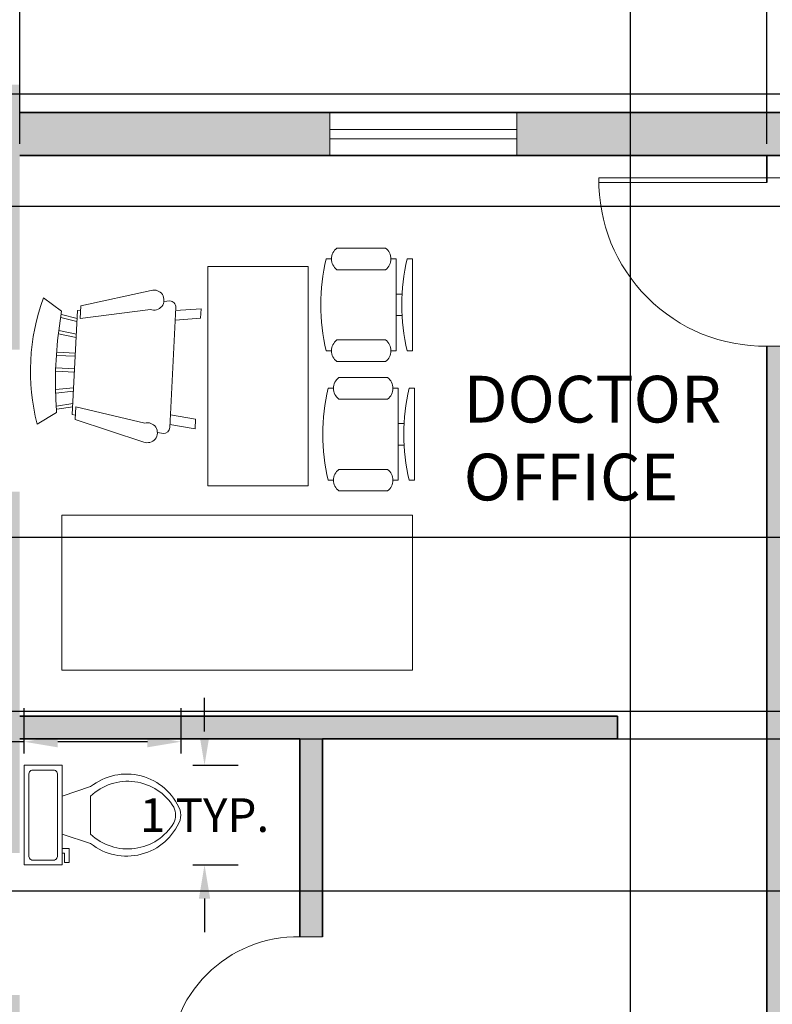
# Model space of a CAD drawing. Units: metres. Extents: x 4298.5 to 4325.2, y 2075 to 2095.8.
# Tile 17 of 35: x 4305.9 to 4309.9, y 2080.5 to 2085.8. Entities that reach past the tile are written whole.
import ezdxf

# ---------------------------------------------------------------- set-up
doc = ezdxf.new("R2010")
doc.units = ezdxf.units.M
for name, color, linetype, lineweight in [('A-ANNO-DIMS', 2, 'Continuous', 18), ('A-AREA-IDEN', 7, 'Continuous', 18), ('A-DOOR', 3, 'Continuous', 18), ('A-EQPM', 9, 'Continuous', 18), ('A-FLOR-FIXT', 15, 'Continuous', 18), ('A-FURN', 15, 'Continuous', 18), ('A-GLAZ', 4, 'Continuous', 18), ('A-WALL', 7, 'Continuous', 35), ('A-WALL-PATT', 252, 'Continuous', 13)]:
    doc.layers.add(name, color=color, linetype=linetype, lineweight=lineweight)
doc.styles.get("Standard").update_dxf_attribs({"font": 'arial.ttf'})
doc.dimstyles.get("Standard").update_dxf_attribs({"dimtxt": 0.18, "dimasz": 0.18, "dimexe": 0.18, "dimexo": 0.0625, "dimgap": 0.09, "dimtad": 0, "dimtih": 1, "dimtoh": 1, "dimdec": 4, "dimzin": 0, "dimdsep": 46, "dimtxsty": 'Standard', "dimcen": 0.09, "dimadec": 0, "dimazin": 0, "dimtfac": 1, "dimtdec": 4, "dimtofl": 0, "dimtmove": 0, "dimatfit": 3, "dimfxl": 1, "dimtolj": 1, "dimtzin": 0, "dimarcsym": 0})

# ---------------------------------------------------------------- blocks, each defined once
blk = doc.blocks.new('Chair - Desk')
for p, q in [((-8.5, 0), (-8.5, -1)), ((-8.5, 0), (8.5, 0)), ((8.5, 0), (8.5, -1)), ((-8.5, -3), (-8.5, -4)), ((-8.5, -3), (8.5, -3)), ((-2, -3), (-2, -1.9355)), ((2, -1.9576), (2, -3)), ((8.5, -3), (8.5, -4)), ((-10.5, -5), (-10.5, -14)), ((-6.5, -14), (-6.5, -5)), ((6.5, -5), (6.5, -14)), ((10.5, -14), (10.5, -5)), ((-8.5, -15), (-8.5, -16)), ((8.5, -15), (8.5, -16))]:
    blk.add_line(p, q)
for centre, radius, start, end in [((0, 34.625), 36.625, 256.5803, 283.4197), ((-8.5, -6.5), 2.5, 36.8699, 143.1301), ((8.5, -6.5), 2.5, 36.8699, 143.1301), ((-8.5, -12.5), 2.5, 216.8699, 323.1301), ((8.5, -12.5), 2.5, 216.8699, 323.1301), ((0, 19.625), 36.625, 256.5803, 283.4197)]:
    blk.add_arc(centre, radius, start, end)
blk = doc.blocks.new('Chair - Rocking')
for p, q in [((-8, -4.5), (-10, -1.5)), ((8, -4.5), (10, -1.5)), ((-7.5, -4.5), (-7, -7)), ((-6.5, -7), (-7.02225, -4.43)), ((-4.5, -7), (-4.96674, -4.19951)), ((-4, -7), (-4.40532, -4.16272)), ((-1.5, -4.05012), (-1.5, -7)), ((-1, -7), (-1, -4.05012)), ((1, -7), (1, -4.04655)), ((1.5, -4.05012), (1.5, -7)), ((4, -7), (4.40187, -4.18694)), ((4.5, -7), (4.96761, -4.19437)), ((6.5, -7), (7, -4.4057)), ((7.5, -4.5), (7, -7)), ((-9, -7.5), (-12, -18.49999)), ((-7, -7.5), (-9, -7.5)), ((-9, -18.49999), (-7, -7.5)), ((-8.23428, -6.99939), (-8.3093, -7.47958)), ((-8.23041, -7), (8.23915, -7)), ((7, -7.5), (9, -7.5)), ((9, -18.49999), (7, -7.5)), ((8.31071, -7.48854), (8.23449, -7.00073)), ((9, -7.5), (12, -18.49999)), ((-10.36644, -20.64523), (-10.5, -21.49999)), ((10.5, -21.49999), (10.3575, -20.58798)), ((-9, -22.49999), (-9.5, -26.49999)), ((0, -22.49999), (-9.5, -22.49999)), ((-8, -26.49999), (-7.5, -22.49999)), ((0, -22.49999), (9.5, -22.49999)), ((8, -26.49999), (7.5, -22.49999)), ((9, -22.49999), (9.5, -26.49999)), ((-9.5, -26.49999), (-8, -26.49999)), ((9.5, -26.49999), (8, -26.49999))]:
    blk.add_line(p, q)
for centre, radius, start, end in [((0, -34.08333), 34.08333, 72.93847, 107.0615), ((0, -68.25004), 64.25, 93.92211, 97.15267), ((0, -68.25004), 64.25, 82.84733, 93.92211), ((-10.5, -18.99999), 1.58114, 161.5651, 18.43495), ((10.5, -18.99999), 1.58114, 161.5651, 18.43495), ((-9.5, -21.49999), 1, 180, 270), ((9.5, -21.49999), 1, 270, 0)]:
    blk.add_arc(centre, radius, start, end)
blk = doc.blocks.new('Toilet - top')
for p, q in [((9.5, -6), (9.5, -2)), ((-8, -8.5), (-8, -8)), ((-7, -8), (-7, -9.5)), ((-4, -8), (-6, -14)), ((4, -8), (6, -14)), ((-10, -8.5), (-8, -8.5)), ((-10, -9.5), (-10, -8.5)), ((-7, -9.5), (-10, -9.5)), ((4, -14), (-4, -14))]:
    blk.add_line(p, q)
blk.add_lwpolyline([(10.5, -8), (10.5, 0), (-10.5, 0), (-10.5, -8)], close=True)
for points in [[(-9.5, -2), (-9.5, -6)], [(8.5, -1), (-8.5, -1)], [(-8.5, -7), (8.5, -7)]]:
    blk.add_lwpolyline(points)
for centre, radius, start, end in [((-8.62, -1.88), 0.884, 81.8699, 188.1301), ((8.62, -1.88), 0.884, 351.8699, 98.1301), ((-8.62, -6.12), 0.884, 171.8699, 278.1301), ((8.62, -6.12), 0.884, 261.8699, 8.1301), ((3.52, -21.58), 12.17, 141.4691, 247.9714), ((4.2, -21.82), 11.33, 136.3677, 238.9468), ((-3.52, -21.58), 12.17, 292.0284, 38.5307), ((-4.2, -21.82), 11.33, 301.053, 43.6321), ((0, -27.88), 4, 245.7318, 294.2682), ((0, -29), 4, 254.8605, 285.1395)]:
    blk.add_arc(centre, radius, start, end)
blk = doc.blocks.new('WIN-1000-GLASS')
for p, q in [((1, 0.05), (0, 0.05)), ((1, 0), (0, 0))]:
    blk.add_line(p, q)
blk = doc.blocks.new('DOOR-900-LEAF')
for p, q in [((0.9, 0.9), (0, 0.9)), ((0.9, 0.875), (0, 0.875))]:
    blk.add_line(p, q)
blk.add_arc((0.8875, 0.8875), 0.8876, 179.1931, 270.8069)
blk = doc.blocks.new('DOOR-700-LEAF')
for p, q in [((0.675, 0), (0.675, 0.7)), ((0.7, 0), (0.7, 0.7))]:
    blk.add_line(p, q)
blk.add_arc((0.6875, 0.0125), 0.6876, 88.9584, 181.0416)
blk = doc.blocks.new('DESK-1175')
blk.add_lwpolyline([(0, 1.1735), (0.5376, 1.1735), (0.5376, 0), (0, 0)], close=True)
blk = doc.blocks.new('EXAM-TABLE-1880')
blk.add_lwpolyline([(0, 0.8289), (1.8779, 0.8289), (1.8779, 0), (0, 0)], close=True)
blk = doc.blocks.new('*D31')
at = {"layer": 'A-ANNO-DIMS', "color": 0, "lineweight": -2, "transparency": 16777216}
for p, q in [((4305.9147, 2081.8585), (4305.9147, 2082.1019)), ((4306.7541, 2081.8585), (4306.7541, 2082.1019)), ((4305.9147, 2081.9219), (4305.7347, 2081.9219)), ((4306.5741, 2081.9219), (4306.0947, 2081.9219))]:
    blk.add_line(p, q, dxfattribs=at)
at = {"layer": 'A-ANNO-DIMS', "color": 0, "transparency": 16777216}
for points in [[(4306.0947, 2081.9519), (4306.0947, 2081.8919), (4305.9147, 2081.9219)], [(4306.5741, 2081.9519), (4306.5741, 2081.8919), (4306.7541, 2081.9219)]]:
    blk.add_solid(points, dxfattribs=at)
at = {"layer": 'Defpoints', "color": 0, "transparency": 16777216}
for p in [(4305.9147, 2081.9219), (4305.9147, 2081.796), (4306.7541, 2081.796)]:
    blk.add_point(p, dxfattribs=at)
at = {"layer": 'A-ANNO-DIMS', "color": 0, "transparency": 16777216, "insert": (4305.0285, 2081.9219), "char_height": 0.18, "attachment_point": 5}
blk.add_mtext('\\A1;WC 1 TYP.', dxfattribs=at)
blk = doc.blocks.new('*D32')
at = {"layer": 'A-ANNO-DIMS', "color": 0, "lineweight": -2, "transparency": 16777216}
for p, q in [((4306.88, 2081.976), (4306.88, 2082.156)), ((4306.8166, 2081.796), (4307.06, 2081.796)), ((4306.8166, 2081.2626), (4307.06, 2081.2626)), ((4306.88, 2081.0826), (4306.88, 2080.9026))]:
    blk.add_line(p, q, dxfattribs=at)
at = {"layer": 'A-ANNO-DIMS', "color": 0, "transparency": 16777216}
for points in [[(4306.85, 2081.976), (4306.91, 2081.976), (4306.88, 2081.796)], [(4306.85, 2081.0826), (4306.91, 2081.0826), (4306.88, 2081.2626)]]:
    blk.add_solid(points, dxfattribs=at)
at = {"layer": 'Defpoints', "color": 0, "transparency": 16777216}
for p in [(4306.7541, 2081.796), (4306.88, 2081.796), (4306.7541, 2081.2626)]:
    blk.add_point(p, dxfattribs=at)
at = {"layer": 'A-ANNO-DIMS', "color": 0, "transparency": 16777216, "insert": (4306.88, 2081.5293), "char_height": 0.18, "attachment_point": 5}
blk.add_mtext('\\A1;1 TYP.', dxfattribs=at)
blk = doc.blocks.new('*D47')
at = {"layer": 'A-ANNO-DIMS', "color": 0, "lineweight": -2, "transparency": 16777216}
for p, q in [((4300.4306, 2084.4956), (4300.4306, 2074.9896)), ((4322.8106, 2084.4956), (4322.8106, 2074.9896)), ((4300.6106, 2075.1696), (4311.2252, 2075.1696)), ((4322.6306, 2075.1696), (4312.016, 2075.1696))]:
    blk.add_line(p, q, dxfattribs=at)
at = {"layer": 'A-ANNO-DIMS', "color": 0, "transparency": 16777216}
for points in [[(4300.6106, 2075.1996), (4300.6106, 2075.1396), (4300.4306, 2075.1696)], [(4322.6306, 2075.1996), (4322.6306, 2075.1396), (4322.8106, 2075.1696)]]:
    blk.add_solid(points, dxfattribs=at)
at = {"layer": 'Defpoints', "color": 0, "transparency": 16777216}
for p in [(4300.4306, 2084.5581), (4322.8106, 2084.5581), (4322.8106, 2075.1696)]:
    blk.add_point(p, dxfattribs=at)
at = {"layer": 'A-ANNO-DIMS', "color": 0, "transparency": 16777216, "insert": (4311.6206, 2075.1696), "char_height": 0.18, "attachment_point": 5}
blk.add_mtext('\\A1;22.38', dxfattribs=at)
blk = doc.blocks.new('*D53')
at = {"layer": 'A-ANNO-DIMS', "color": 0, "lineweight": -2, "transparency": 16777216}
for p, q in [((4309.1606, 2076.3906), (4309.1606, 2095.8166)), ((4316.8106, 2076.3906), (4316.8106, 2095.8166)), ((4309.3406, 2095.6366), (4312.6619, 2095.6366)), ((4316.6306, 2095.6366), (4313.3093, 2095.6366))]:
    blk.add_line(p, q, dxfattribs=at)
at = {"layer": 'A-ANNO-DIMS', "color": 0, "transparency": 16777216}
for points in [[(4309.3406, 2095.6666), (4309.3406, 2095.6066), (4309.1606, 2095.6366)], [(4316.6306, 2095.6666), (4316.6306, 2095.6066), (4316.8106, 2095.6366)]]:
    blk.add_solid(points, dxfattribs=at)
at = {"layer": 'Defpoints', "color": 0, "transparency": 16777216}
for p in [(4316.8106, 2095.6366), (4309.1606, 2076.3281), (4316.8106, 2076.3281)]:
    blk.add_point(p, dxfattribs=at)
at = {"layer": 'A-ANNO-DIMS', "color": 0, "transparency": 16777216, "insert": (4312.9856, 2095.6366), "char_height": 0.18, "attachment_point": 5}
blk.add_mtext('\\A1;7.65', dxfattribs=at)
blk = doc.blocks.new('*D56')
at = {"layer": 'A-ANNO-DIMS', "color": 0, "lineweight": -2, "transparency": 16777216}
for p, q in [((4305.8281, 2085.0581), (4299.0921, 2085.0581)), ((4299.2721, 2084.8781), (4299.2721, 2083.74)), ((4299.2721, 2082.2381), (4299.2721, 2083.3761)), ((4305.8281, 2082.0581), (4299.0921, 2082.0581))]:
    blk.add_line(p, q, dxfattribs=at)
at = {"layer": 'A-ANNO-DIMS', "color": 0, "transparency": 16777216}
for points in [[(4299.2421, 2084.8781), (4299.3021, 2084.8781), (4299.2721, 2085.0581)], [(4299.2421, 2082.2381), (4299.3021, 2082.2381), (4299.2721, 2082.0581)]]:
    blk.add_solid(points, dxfattribs=at)
at = {"layer": 'Defpoints', "color": 0, "transparency": 16777216}
for p in [(4299.2721, 2085.0581), (4305.8906, 2085.0581), (4305.8906, 2082.0581)]:
    blk.add_point(p, dxfattribs=at)
at = {"layer": 'A-ANNO-DIMS', "color": 0, "transparency": 16777216, "insert": (4299.2721, 2083.5581), "char_height": 0.18, "attachment_point": 5}
blk.add_mtext('\\A1;3', dxfattribs=at)
blk = doc.blocks.new('*D57')
at = {"layer": 'A-ANNO-DIMS', "color": 0, "lineweight": -2, "transparency": 16777216}
for p, q in [((4305.8906, 2085.1206), (4305.8906, 2095.8166)), ((4309.8906, 2085.1206), (4309.8906, 2095.8166)), ((4306.0706, 2095.6366), (4307.7383, 2095.6366)), ((4309.7106, 2095.6366), (4308.0428, 2095.6366))]:
    blk.add_line(p, q, dxfattribs=at)
at = {"layer": 'A-ANNO-DIMS', "color": 0, "transparency": 16777216}
for points in [[(4306.0706, 2095.6666), (4306.0706, 2095.6066), (4305.8906, 2095.6366)], [(4309.7106, 2095.6666), (4309.7106, 2095.6066), (4309.8906, 2095.6366)]]:
    blk.add_solid(points, dxfattribs=at)
at = {"layer": 'Defpoints', "color": 0, "transparency": 16777216}
for p in [(4309.8906, 2095.6366), (4305.8906, 2085.0581), (4309.8906, 2085.0581)]:
    blk.add_point(p, dxfattribs=at)
at = {"layer": 'A-ANNO-DIMS', "color": 0, "transparency": 16777216, "insert": (4307.8906, 2095.6366), "char_height": 0.18, "attachment_point": 5}
blk.add_mtext('\\A1;4', dxfattribs=at)
blk = doc.blocks.new('*D58')
at = {"layer": 'A-ANNO-DIMS', "color": 0, "lineweight": -2, "transparency": 16777216}
for p, q in [((4324.5871, 2085.3881), (4324.5871, 2085.5681)), ((4324.5871, 2085.5681), (4324.7671, 2085.5681)), ((4300.7231, 2085.3881), (4324.7671, 2085.3881)), ((4324.5871, 2084.9681), (4324.5871, 2085.2081)), ((4300.7231, 2084.7881), (4324.7671, 2084.7881))]:
    blk.add_line(p, q, dxfattribs=at)
at = {"layer": 'A-ANNO-DIMS', "color": 0, "transparency": 16777216}
for points in [[(4324.5571, 2085.2081), (4324.6171, 2085.2081), (4324.5871, 2085.3881)], [(4324.5571, 2084.9681), (4324.6171, 2084.9681), (4324.5871, 2084.7881)]]:
    blk.add_solid(points, dxfattribs=at)
at = {"layer": 'Defpoints', "color": 0, "transparency": 16777216}
for p in [(4300.6606, 2085.3881), (4324.5871, 2085.3881), (4300.6606, 2084.7881)]:
    blk.add_point(p, dxfattribs=at)
at = {"layer": 'A-ANNO-DIMS', "color": 0, "transparency": 16777216, "insert": (4325.0209, 2085.5681), "char_height": 0.18, "attachment_point": 5}
blk.add_mtext('\\A1;0.6', dxfattribs=at)
blk = doc.blocks.new('*D60')
at = {"layer": 'A-ANNO-DIMS', "color": 0, "lineweight": -2, "transparency": 16777216}
for p, q in [((4305.9531, 2081.9381), (4324.7671, 2081.9381)), ((4324.5871, 2081.7581), (4324.5871, 2081.18)), ((4324.5871, 2080.2381), (4324.5871, 2080.8162)), ((4305.9531, 2080.0581), (4324.7671, 2080.0581))]:
    blk.add_line(p, q, dxfattribs=at)
at = {"layer": 'A-ANNO-DIMS', "color": 0, "transparency": 16777216}
for points in [[(4324.5571, 2081.7581), (4324.6171, 2081.7581), (4324.5871, 2081.9381)], [(4324.5571, 2080.2381), (4324.6171, 2080.2381), (4324.5871, 2080.0581)]]:
    blk.add_solid(points, dxfattribs=at)
at = {"layer": 'Defpoints', "color": 0, "transparency": 16777216}
for p in [(4305.8906, 2081.9381), (4324.5871, 2081.9381), (4305.8906, 2080.0581)]:
    blk.add_point(p, dxfattribs=at)
at = {"layer": 'A-ANNO-DIMS', "color": 0, "transparency": 16777216, "insert": (4324.5871, 2080.9981), "char_height": 0.18, "attachment_point": 5}
blk.add_mtext('\\A1;1.88', dxfattribs=at)
blk = doc.blocks.new('*D62')
at = {"layer": 'A-ANNO-DIMS', "color": 0, "lineweight": -2, "transparency": 16777216}
for p, q in [((4312.1097, 2083.0153), (4299.0921, 2083.0153)), ((4299.2721, 2082.8353), (4299.2721, 2082.7313)), ((4299.2721, 2082.2635), (4299.2721, 2082.3674)), ((4312.1097, 2082.0835), (4299.0921, 2082.0835))]:
    blk.add_line(p, q, dxfattribs=at)
at = {"layer": 'A-ANNO-DIMS', "color": 0, "transparency": 16777216}
for points in [[(4299.2421, 2082.8353), (4299.3021, 2082.8353), (4299.2721, 2083.0153)], [(4299.2421, 2082.2635), (4299.3021, 2082.2635), (4299.2721, 2082.0835)]]:
    blk.add_solid(points, dxfattribs=at)
at = {"layer": 'Defpoints', "color": 0, "transparency": 16777216}
for p in [(4312.1722, 2083.0153), (4299.2721, 2082.0835), (4312.1722, 2082.0835)]:
    blk.add_point(p, dxfattribs=at)
at = {"layer": 'A-ANNO-DIMS', "color": 0, "transparency": 16777216, "insert": (4299.2721, 2082.5494), "char_height": 0.18, "attachment_point": 5}
blk.add_mtext('\\A1;0.93', dxfattribs=at)
blk = doc.blocks.new('*D63')
at = {"layer": 'A-ANNO-DIMS', "color": 0, "lineweight": -2, "transparency": 16777216}
for p, q in [((4312.1097, 2082.0835), (4299.0921, 2082.0835)), ((4299.2721, 2081.9035), (4299.2721, 2081.7847)), ((4299.2721, 2081.3021), (4299.2721, 2081.4209)), ((4312.1097, 2081.1221), (4299.0921, 2081.1221))]:
    blk.add_line(p, q, dxfattribs=at)
at = {"layer": 'A-ANNO-DIMS', "color": 0, "transparency": 16777216}
for points in [[(4299.2421, 2081.9035), (4299.3021, 2081.9035), (4299.2721, 2082.0835)], [(4299.2421, 2081.3021), (4299.3021, 2081.3021), (4299.2721, 2081.1221)]]:
    blk.add_solid(points, dxfattribs=at)
at = {"layer": 'Defpoints', "color": 0, "transparency": 16777216}
for p in [(4312.1722, 2082.0835), (4299.2721, 2081.1221), (4312.1722, 2081.1221)]:
    blk.add_point(p, dxfattribs=at)
at = {"layer": 'A-ANNO-DIMS', "color": 0, "transparency": 16777216, "insert": (4299.2721, 2081.6028), "char_height": 0.18, "attachment_point": 5}
blk.add_mtext('\\A1;0.96', dxfattribs=at)
blk = doc.blocks.new('*D64')
at = {"layer": 'A-ANNO-DIMS', "color": 0, "lineweight": -2, "transparency": 16777216}
for p, q in [((4312.1097, 2081.1221), (4299.0921, 2081.1221)), ((4299.2721, 2080.9421), (4299.2721, 2080.427)), ((4312.1097, 2080.247), (4299.0921, 2080.247)), ((4299.2721, 2080.247), (4299.2721, 2080.067)), ((4299.2721, 2080.067), (4299.0921, 2080.067))]:
    blk.add_line(p, q, dxfattribs=at)
at = {"layer": 'A-ANNO-DIMS', "color": 0, "transparency": 16777216}
for points in [[(4299.2421, 2080.9421), (4299.3021, 2080.9421), (4299.2721, 2081.1221)], [(4299.2421, 2080.427), (4299.3021, 2080.427), (4299.2721, 2080.247)]]:
    blk.add_solid(points, dxfattribs=at)
at = {"layer": 'Defpoints', "color": 0, "transparency": 16777216}
for p in [(4312.1722, 2081.1221), (4299.2721, 2080.247), (4312.1722, 2080.247)]:
    blk.add_point(p, dxfattribs=at)
at = {"layer": 'A-ANNO-DIMS', "color": 0, "transparency": 16777216, "insert": (4298.7681, 2080.067), "char_height": 0.18, "attachment_point": 5}
blk.add_mtext('\\A1;0.88', dxfattribs=at)

msp = doc.modelspace()

# ---------------------------------------------------------------- hatches: boundary and pattern name
at = {"layer": 'A-WALL-PATT'}
h = msp.add_hatch(color=256, dxfattribs=at)
h.dxf.hatch_style = 1
h.paths.add_polyline_path([(4308.7606, 2094.4781), (4308.1606, 2094.4781), (4307.4606, 2094.4781), (4307.4606, 2094.2481), (4308.2706, 2094.2481), (4308.2706, 2094.1281), (4308.3906, 2094.1281), (4308.3906, 2094.2481), (4308.7606, 2094.2481)])
h.paths.add_polyline_path([(4310.1206, 2094.4781), (4309.5206, 2094.4781), (4309.5206, 2094.2481), (4309.8906, 2094.2481), (4309.8906, 2092.2481), (4308.3906, 2092.2481), (4308.3906, 2093.4281), (4308.2706, 2093.4281), (4308.2706, 2092.0181), (4309.8906, 2092.0181), (4309.8906, 2087.0181), (4309.7706, 2087.0181), (4309.7706, 2086.7881), (4309.8906, 2086.7881), (4311.9406, 2086.7881), (4311.9406, 2087.0181), (4310.1206, 2087.0181), (4310.1206, 2089.0181), (4310.2406, 2089.0181), (4310.2406, 2089.1381), (4310.1206, 2089.1381), (4310.1206, 2092.0181), (4310.3078, 2092.0181), (4310.3078, 2092.2481), (4310.1206, 2092.2481)])
h.paths.add_polyline_path([(4311.7406, 2092.2481), (4311.0678, 2092.2481), (4311.0678, 2092.0181), (4311.7406, 2092.0181)], flags=17)
h.paths.add_polyline_path([(4313.1733, 2092.2481), (4312.5006, 2092.2481), (4312.5006, 2092.0181), (4313.1733, 2092.0181)])
h.paths.add_polyline_path([(4314.5378, 2092.2481), (4314.1206, 2092.2481), (4313.9333, 2092.2481), (4313.9333, 2092.0181), (4314.1206, 2092.0181), (4314.1206, 2087.0181), (4314.0006, 2087.0181), (4314.0006, 2086.7881), (4314.1206, 2086.7881), (4315.5718, 2086.7881), (4315.5718, 2087.0181), (4314.3506, 2087.0181), (4314.3506, 2092.0181), (4314.5378, 2092.0181)])
h.paths.add_polyline_path([(4315.9706, 2092.2481), (4315.2978, 2092.2481), (4315.2978, 2092.0181), (4315.9706, 2092.0181)])
h.paths.add_polyline_path([(4317.4033, 2092.2481), (4316.7306, 2092.2481), (4316.7306, 2092.0181), (4317.4033, 2092.0181)])
h.paths.add_polyline_path([(4318.9506, 2092.2481), (4318.3506, 2092.2481), (4318.1633, 2092.2481), (4318.1633, 2092.0181), (4318.3506, 2092.0181), (4318.3506, 2091.8981), (4318.5806, 2091.8981), (4318.5806, 2092.0181), (4318.9506, 2092.0181)])
h.paths.add_polyline_path([(4321.0106, 2092.2481), (4319.7106, 2092.2481), (4319.7106, 2092.0181), (4320.0806, 2092.0181), (4320.0806, 2090.0181), (4318.5806, 2090.0181), (4318.5806, 2091.1981), (4318.3506, 2091.1981), (4318.3506, 2090.0181), (4318.3506, 2087.0181), (4318.2306, 2087.0181), (4318.2306, 2086.7881), (4318.3506, 2086.7881), (4318.3506, 2086.3081), (4318.5806, 2086.3081), (4318.5806, 2089.7881), (4321.7806, 2089.7881), (4321.7806, 2090.0181), (4320.2006, 2090.0181), (4320.2006, 2092.0181), (4321.0106, 2092.0181)])
h.paths.add_polyline_path([(4322.8106, 2092.2481), (4321.7706, 2092.2481), (4321.7706, 2092.0181), (4322.5806, 2092.0181), (4322.5806, 2091.2831), (4322.8106, 2091.2831)])
h.paths.add_polyline_path([(4322.8106, 2090.5231), (4322.5806, 2090.5231), (4322.5806, 2089.7881), (4322.5806, 2089.5254), (4322.8106, 2089.5254), (4322.8106, 2090.0181)])
h.paths.add_polyline_path([(4322.8106, 2088.7654), (4322.5806, 2088.7654), (4322.5806, 2087.6681), (4322.8106, 2087.6681)])
h.paths.add_polyline_path([(4322.8106, 2086.9081), (4322.5806, 2086.9081), (4322.5806, 2085.8107), (4322.8106, 2085.8107)])
h.paths.add_polyline_path([(4322.8106, 2085.0507), (4322.5806, 2085.0507), (4322.5806, 2084.7881), (4318.5806, 2084.7881), (4318.5806, 2085.0581), (4318.5806, 2085.4081), (4318.3506, 2085.4081), (4318.3506, 2084.5581), (4318.3506, 2080.8581), (4318.4706, 2080.8581), (4318.4706, 2082.3281), (4319.2606, 2082.3281), (4319.2606, 2082.5581), (4318.5806, 2082.5581), (4318.5806, 2084.5581), (4320.0806, 2084.5581), (4320.0806, 2083.9381), (4320.3106, 2083.9381), (4320.3106, 2084.5581), (4322.8106, 2084.5581)])
h.paths.add_polyline_path([(4320.3106, 2083.1781), (4320.0806, 2083.1781), (4320.0806, 2082.5581), (4319.9606, 2082.5581), (4319.9606, 2082.3281), (4320.0806, 2082.3281), (4320.0806, 2081.5731), (4320.3106, 2081.5731)], flags=17)
h.paths.add_polyline_path([(4320.3106, 2080.8131), (4320.0806, 2080.8131), (4320.0806, 2080.0581), (4318.4286, 2080.0581), (4318.4286, 2079.8281), (4320.3106, 2079.8281)])
h.paths.add_polyline_path([(4317.3506, 2085.2881), (4316.5718, 2085.2881), (4316.5718, 2085.0581), (4317.3506, 2085.0581)])
h.paths.add_polyline_path([(4315.5718, 2085.2881), (4314.8434, 2085.2881), (4314.8434, 2085.0581), (4315.5718, 2085.0581)])
h.paths.add_polyline_path([(4313.8434, 2085.2881), (4312.9406, 2085.2881), (4312.9406, 2085.0581), (4313.8434, 2085.0581)])
h.paths.add_polyline_path([(4311.9406, 2085.2881), (4311.4406, 2085.2881), (4311.4406, 2085.0581), (4311.9406, 2085.0581)])
h.paths.add_polyline_path([(4317.3306, 2087.0181), (4316.5718, 2087.0181), (4316.5718, 2086.7881), (4317.3306, 2086.7881)])
h.paths.add_polyline_path([(4313.1006, 2089.1381), (4311.1406, 2089.1381), (4311.1406, 2089.0181), (4312.9806, 2089.0181), (4312.9806, 2087.0181), (4312.9406, 2087.0181), (4312.9406, 2086.7881), (4313.1006, 2086.7881), (4313.1006, 2087.0181)])
h.paths.add_polyline_path([(4307.5515, 2087.0181), (4305.8906, 2087.0181), (4305.8906, 2092.2481), (4305.8906, 2094.2481), (4306.7006, 2094.2481), (4306.7006, 2094.4781), (4305.6606, 2094.4781), (4305.6606, 2092.2481), (4305.2906, 2092.2481), (4305.2906, 2092.0181), (4305.6606, 2092.0181), (4305.6606, 2090.0181), (4304.1606, 2090.0181), (4304.1606, 2091.1981), (4304.0406, 2091.1981), (4304.0406, 2089.9081), (4301.5606, 2089.9081), (4301.5606, 2089.7881), (4304.0406, 2089.7881), (4305.6606, 2089.7881), (4305.6606, 2086.6381), (4305.8906, 2086.6381), (4305.8906, 2086.7881), (4307.5515, 2086.7881)])
h.paths.add_polyline_path([(4307.5515, 2085.2881), (4305.8906, 2085.2881), (4305.8906, 2085.4381), (4305.6606, 2085.4381), (4305.6606, 2084.7881), (4305.2906, 2084.7881), (4305.2906, 2084.5581), (4305.6606, 2084.5581), (4305.6606, 2084.02), (4305.8906, 2084.02), (4305.8906, 2084.5581), (4305.8906, 2085.0581), (4307.5515, 2085.0581)])
h.paths.add_polyline_path([(4310.2406, 2085.2881), (4308.5515, 2085.2881), (4308.5515, 2085.0581), (4310.2406, 2085.0581)])
h.paths.add_polyline_path([(4317.4286, 2080.0581), (4316.5718, 2080.0581), (4316.5718, 2079.8281), (4317.4286, 2079.8281)])
h.paths.add_polyline_path([(4315.5718, 2080.0581), (4314.8434, 2080.0581), (4314.8434, 2079.8281), (4315.5718, 2079.8281)])
h.paths.add_polyline_path([(4313.8434, 2080.0581), (4312.9406, 2080.0581), (4312.9406, 2079.8281), (4313.8434, 2079.8281)])
h.paths.add_polyline_path([(4311.9406, 2080.0581), (4311.4406, 2080.0581), (4311.4406, 2079.8281), (4311.9406, 2079.8281)])
h.paths.add_polyline_path([(4310.2406, 2080.0581), (4310.1206, 2080.0581), (4310.1206, 2084.0381), (4309.8906, 2084.0381), (4309.8906, 2080.0581), (4309.1606, 2080.0581), (4309.1606, 2079.8281), (4310.2406, 2079.8281)])
h.paths.add_polyline_path([(4308.1606, 2080.0581), (4307.5106, 2080.0581), (4307.5106, 2080.1781), (4307.3906, 2080.1781), (4307.3906, 2080.0581), (4305.8906, 2080.0581), (4305.8906, 2080.567), (4305.6606, 2080.567), (4305.6606, 2079.8281), (4308.1606, 2079.8281)])
h.paths.add_polyline_path([(4307.5106, 2081.9381), (4309.0906, 2081.9381), (4309.0906, 2082.0581), (4305.8906, 2082.0581), (4305.8906, 2083.26), (4305.6606, 2083.26), (4305.6606, 2081.327), (4305.8906, 2081.327), (4305.8906, 2081.9381), (4307.3906, 2081.9381), (4307.3906, 2080.8781), (4307.5106, 2080.8781)])
h.paths.add_polyline_path([(4304.5306, 2084.7881), (4302.7306, 2084.7881), (4302.7306, 2084.5581), (4304.5306, 2084.5581)])
h.paths.add_polyline_path([(4301.9706, 2084.7881), (4300.6606, 2084.7881), (4300.6606, 2085.0249), (4300.4306, 2085.0249), (4300.4306, 2084.5581), (4301.9706, 2084.5581)])
h.paths.add_polyline_path([(4300.6606, 2086.8843), (4300.4306, 2086.8843), (4300.4306, 2085.7849), (4300.6606, 2085.7849)])
h.paths.add_polyline_path([(4300.6606, 2089.1618), (4300.4306, 2089.1618), (4300.4306, 2087.6443), (4300.6606, 2087.6443)])
h.paths.add_polyline_path([(4300.6606, 2091.0212), (4300.4306, 2091.0212), (4300.4306, 2089.9218), (4300.6606, 2089.9218)])
h.paths.add_polyline_path([(4300.6606, 2092.0181), (4301.9706, 2092.0181), (4301.9706, 2092.2481), (4300.4306, 2092.2481), (4300.4306, 2091.7812), (4300.6606, 2091.7812)])
h.paths.add_polyline_path([(4304.5306, 2092.2481), (4302.7306, 2092.2481), (4302.7306, 2092.0181), (4304.0406, 2092.0181), (4304.0406, 2091.8981), (4304.1606, 2091.8981), (4304.1606, 2092.0181), (4304.5306, 2092.0181)], flags=17)

# ---------------------------------------------------------------- linework, layer by layer
at = {"layer": 'A-DOOR'}
for p, q in [((4309.8906, 2084.9381), (4310.1206, 2084.9381)), ((4309.8906, 2084.0381), (4310.1206, 2084.0381)), ((4307.3906, 2080.8781), (4307.5106, 2080.8781))]:
    msp.add_line(p, q, dxfattribs=at)
at = {"layer": 'A-GLAZ'}
for p, q in [((4307.5515, 2085.0581), (4307.5515, 2085.2881)), ((4308.5515, 2085.0581), (4308.5515, 2085.2881))]:
    msp.add_line(p, q, dxfattribs=at)
at = {"layer": 'A-WALL'}
for p, q in [((4305.8906, 2085.2881), (4310.2406, 2085.2881)), ((4305.8906, 2085.0581), (4310.2406, 2085.0581)), ((4309.8906, 2085.0581), (4309.8906, 2084.9131)), ((4309.8906, 2084.0381), (4309.8906, 2080.0581)), ((4305.8906, 2082.0581), (4309.0906, 2082.0581)), ((4309.0906, 2081.9381), (4309.0906, 2082.0581)), ((4305.8906, 2081.9381), (4307.3906, 2081.9381)), ((4307.3906, 2081.9381), (4307.3906, 2080.8781)), ((4307.5106, 2081.9381), (4307.5106, 2080.8781)), ((4307.5106, 2081.9381), (4309.0906, 2081.9381))]:
    msp.add_line(p, q, dxfattribs=at)

# ---------------------------------------------------------------- block references
at = {"layer": 'A-DOOR'}
msp.add_blockref('DOOR-900-LEAF', (4308.9906, 2084.0381), dxfattribs=at)
at = {"layer": 'A-DOOR', "extrusion": (0, 0, -1), "zscale": -1, "rotation": 270.0000000000699}
msp.add_blockref('DOOR-700-LEAF', (-4307.3906, 2080.8781), dxfattribs=at)
at = {"layer": 'A-EQPM'}
msp.add_blockref('EXAM-TABLE-1880', (4306.116, 2082.305), dxfattribs=at)
at = {"layer": 'A-FLOR-FIXT', "xscale": 0.0254, "yscale": 0.0254, "zscale": 0.0254, "rotation": 90.00004036649993}
msp.add_blockref('Toilet - top', (4305.9147, 2081.5293), dxfattribs=at)
at = {"layer": 'A-FURN'}
for name, p, xscale, yscale, zscale, rotation in [('Chair - Desk', (4307.9931, 2084.2593), 0.0288995186862949, 0.0288995186862949, 0.0288995186862949, 270), ('Chair - Rocking', (4305.9497, 2083.9621), 0.0338365474760119, 0.0338365474760119, 0.0338365474760119, 87.13759363081944), ('Chair - Desk', (4308.0038, 2083.567), 0.0288995186862949, 0.0288995186862949, 0.0288995186862949, 270)]:
    msp.add_blockref(name, p, dxfattribs=dict(at, xscale=xscale, yscale=yscale, zscale=zscale, rotation=rotation))
msp.add_blockref('DESK-1175', (4306.8976, 2083.2908), dxfattribs=at)
at = {"layer": 'A-GLAZ', "rotation": 180}
msp.add_blockref('WIN-1000-GLASS', (4308.5515, 2085.1981), dxfattribs=at)

# ---------------------------------------------------------------- texts
at = {"layer": 'A-AREA-IDEN', "insert": (4308.2673, 2083.8797), "char_height": 0.25, "attachment_point": 1}
msp.add_mtext_dynamic_manual_height_columns('DOCTOR OFFICE', width=2.22034, gutter_width=12.5, heights=[0], dxfattribs=at)

# ---------------------------------------------------------------- dimensions: what is measured, and where the dimension line sits
at = {"layer": 'A-ANNO-DIMS'}
for base, p1, p2, override, picture, middle in [((4309.8906, 2095.6366), (4305.8906, 2085.0581), (4309.8906, 2085.0581), {"dimdec": 0, "dimlfac": 1, "dimrnd": 0, "dimzin": 0, "dimdsep": 46, "dimlunit": 2}, '*D57', (4307.8906, 2095.6366)), ((4316.8106, 2095.6366), (4309.1606, 2076.3281), (4316.8106, 2076.3281), {"dimdec": 2, "dimlfac": 1, "dimrnd": 0, "dimzin": 0, "dimdsep": 46, "dimlunit": 2}, '*D53', (4312.9856, 2095.6366)), ((4322.8106, 2075.1696), (4300.4306, 2084.5581), (4322.8106, 2084.5581), {"dimdec": 2, "dimlfac": 1, "dimrnd": 0, "dimzin": 0, "dimdsep": 46, "dimlunit": 2}, '*D47', (4311.6206, 2075.1696))]:
    dim = msp.add_linear_dim(base=base, p1=p1, p2=p2, dimstyle='Standard', override=override, dxfattribs=at)
    dim.commit()
    dim.dimension.update_dxf_attribs({"geometry": picture, "text_midpoint": middle})
for base, p1, p2, override, picture, middle in [((4324.5871, 2085.3881), (4300.6606, 2084.7881), (4300.6606, 2085.3881), {"dimdec": 1, "dimlfac": 1, "dimrnd": 0, "dimzin": 0, "dimdsep": 46, "dimlunit": 2}, '*D58', (4325.0209, 2085.5681)), ((4299.2721, 2085.0581), (4305.8906, 2082.0581), (4305.8906, 2085.0581), {"dimdec": 0, "dimlfac": 1, "dimrnd": 0, "dimzin": 0, "dimdsep": 46, "dimlunit": 2}, '*D56', (4299.2721, 2083.5581)), ((4299.2721, 2082.0835), (4312.1722, 2083.0153), (4312.1722, 2082.0835), {"dimdec": 2, "dimlfac": 1, "dimrnd": 0, "dimzin": 0, "dimdsep": 46, "dimlunit": 2}, '*D62', (4299.2721, 2082.5494)), ((4299.2721, 2081.1221), (4312.1722, 2082.0835), (4312.1722, 2081.1221), {"dimdec": 2, "dimlfac": 1, "dimrnd": 0, "dimzin": 0, "dimdsep": 46, "dimlunit": 2}, '*D63', (4299.2721, 2081.6028)), ((4324.5871, 2081.9381), (4305.8906, 2080.0581), (4305.8906, 2081.9381), {"dimdec": 2, "dimlfac": 1, "dimrnd": 0, "dimzin": 0, "dimdsep": 46, "dimlunit": 2}, '*D60', (4324.5871, 2080.9981)), ((4299.2721, 2080.247), (4312.1722, 2081.1221), (4312.1722, 2080.247), {"dimdec": 2, "dimlfac": 1, "dimrnd": 0, "dimzin": 0, "dimdsep": 46, "dimlunit": 2}, '*D64', (4298.7681, 2080.067))]:
    dim = msp.add_linear_dim(base=base, p1=p1, p2=p2, angle=90, dimstyle='Standard', override=override, dxfattribs=at)
    dim.commit()
    dim.dimension.update_dxf_attribs({"geometry": picture, "text_midpoint": middle})
for base, p1, p2, angle, text, picture, middle in [((4305.9147, 2081.9219), (4306.7541, 2081.796), (4305.9147, 2081.796), 180, 'WC <> TYP.', '*D31', (4305.0285, 2081.9219)), ((4306.88, 2081.796), (4306.7541, 2081.2626), (4306.7541, 2081.796), 90, '<> TYP.', '*D32', (4306.88, 2081.5293))]:
    dim = msp.add_linear_dim(base=base, p1=p1, p2=p2, angle=angle, text=text, dimstyle='Standard', override={"dimdec": 0, "dimlfac": 1, "dimrnd": 0, "dimzin": 0, "dimdsep": 46, "dimlunit": 2}, dxfattribs=at)
    dim.commit()
    dim.dimension.update_dxf_attribs({"geometry": picture, "text_midpoint": middle})

doc.saveas('drawing.dxf')
